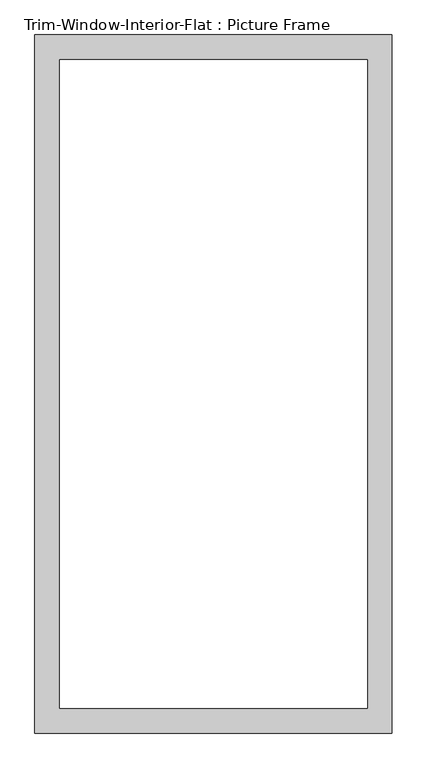
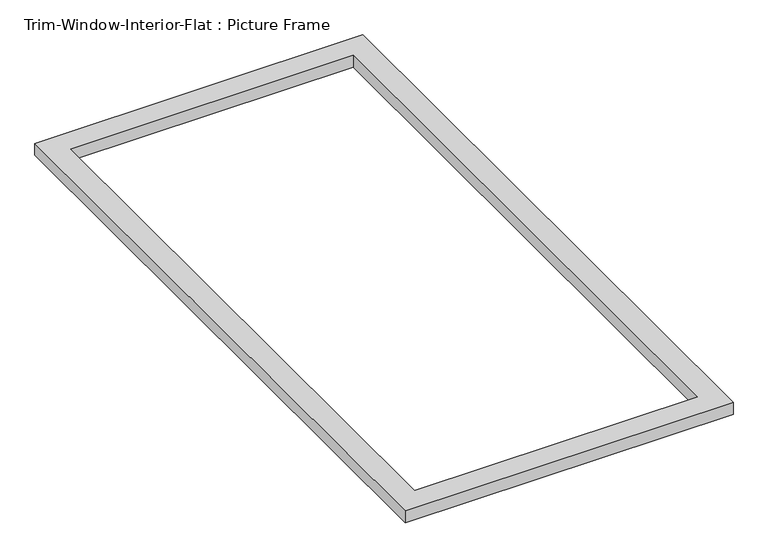
"""IFC4 building model written with IfcOpenShell, lengths in millimetres: proxy geometry, Trim-Window-Interior-Flat : Picture Frame."""

from ifc_helpers import new_model, si_unit, origin, origin_with_axes, place, context, project, spatial, polyline, outline, extrude, source, transform, mapped, element, save


def trim_window_interior_flat_picture_frame_4c1e0c81(model_context):
    return source(origin(), model_context, "Body", "SweptSolid", [
        extrude(outline(polyline([(412.75, 44.45), (412.75, -1568.45), (-412.75, -1568.45), (-412.75, 44.45), (412.75, 44.45)]), holes=[polyline([(355.6, -12.7), (-355.6, -12.7), (-355.6, -1511.3), (355.6, -1511.3), (355.6, -12.7)])]), origin_with_axes(), (0.0, 0.0, 1.0), 31.75),
    ])


if __name__ == "__main__":
    model = new_model("IFC4")
    model_context = context("Model", 3, world=origin())
    ifc_project = project(units=[si_unit("LENGTHUNIT", "METRE", prefix="MILLI")], contexts=[model_context])
    site = spatial("IfcSite", under=ifc_project)
    building = spatial("IfcBuilding", under=site)
    placement = place(None, origin())
    trim_window_interior_flat_picture_frame_shape = trim_window_interior_flat_picture_frame_4c1e0c81(model_context)
    element("IfcBuildingElementProxy", 1, Name="Trim-Window-Interior-Flat : Picture Frame", ObjectType="Trim-Window-Interior-Flat : Picture Frame", at=placement, inside=building, context=model_context, shape_type="MappedRepresentation", body=[
        mapped(trim_window_interior_flat_picture_frame_shape, transform((0.0, 0.0, 0.0), x_axis=(1.0, 0.0, 0.0), y_axis=(0.0, 1.0, 0.0), z_axis=(0.0, 0.0, 1.0))),
    ])
    save(model, "model.ifc")

# Revit data of these elements
# Type "Trim-Window-Interior-Flat : Picture Frame"
#   Trim Thickness_Picture Frame = 0' - 1 1/4"
#   Trim Width = 0' - 2 1/4"
#   Trim Thickness_with Sill = 0' - 0 3/4"
#   Sill Thickness = 0' - 1 1/4"
#   Opening Width [instance default] = 2' - 0"
#   Opening Height [instance default] = 3' - 0"
#   Default Elevation = 4' - 0"
#   Sill = no
#   Picture Frame = yes
#   Trim Material [instance default] = none
# Element 1 (IfcBuildingElementProxy, "Trim-Window-Interior-Flat : Picture Frame")
#   Opening Width = 2' - 5"
#   Opening Height = 5' - 0"
#   Trim Material = Wood - Stained
#   Materials on its faces: "Wood - Stained"
# Materials
#   "Wood - Stained": class "Wood", colour RGB 224 178 126, transparency 0, Cost = 0
